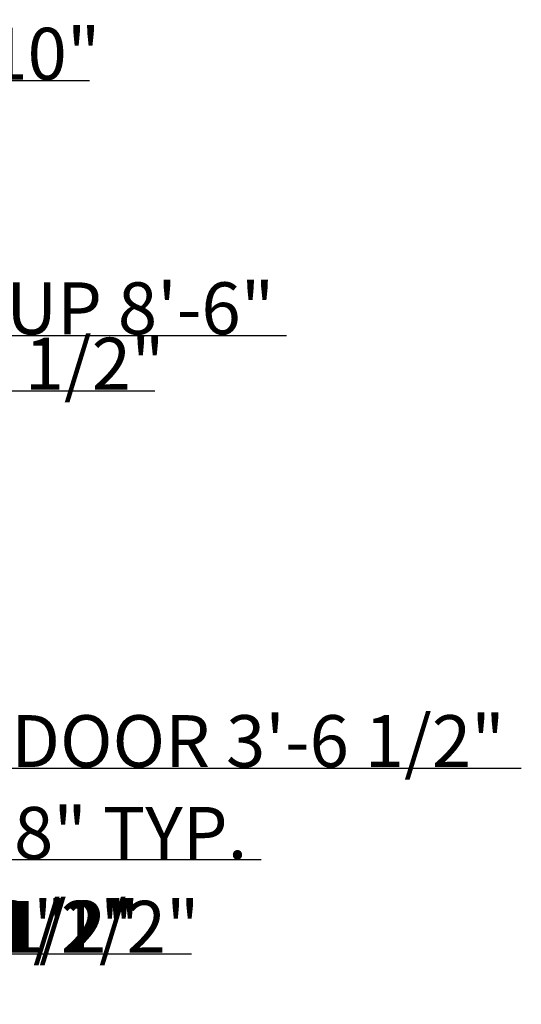
# Model space of a CAD drawing. Units: inches. Extents: x 2236 to 2927, y 1577 to 2452.
# Tile 8 of 9: x 2695 to 2927, y 1679 to 2134. Entities that reach past the tile are written whole.
import ezdxf

# ---------------------------------------------------------------- set-up
doc = ezdxf.new("R2010")
doc.units = ezdxf.units.IN
doc.layers.add('A-ANNO-DIMS', color=2, linetype='Continuous', lineweight=18)
doc.styles.get("Standard").update_dxf_attribs({"font": 'arial.ttf'})
doc.dimstyles.get("Standard").update_dxf_attribs({"dimtxt": 24, "dimasz": 12, "dimexe": 0.18, "dimexo": 0.0625, "dimgap": 0.09, "dimtad": 1, "dimdec": 1, "dimzin": 0, "dimdsep": 46, "dimlunit": 4, "dimtxsty": 'Standard', "dimcen": 0.09, "dimadec": 0, "dimazin": 0, "dimtfac": 1, "dimtdec": 1, "dimtofl": 0, "dimtmove": 0, "dimatfit": 3, "dimfxl": 1, "dimtolj": 1, "dimtzin": 0, "dimarcsym": 0})

# ---------------------------------------------------------------- blocks, each defined once
blk = doc.blocks.new('*D24')
at = {"layer": 'A-ANNO-DIMS', "color": 0, "lineweight": -2, "transparency": 16777216}
for p, q in [((2478.46, 1747), (2478.46, 1745.71)), ((2486.29, 1747), (2486.29, 1745.71)), ((2466.46, 1745.89), (2454.46, 1745.89)), ((2498.29, 1745.89), (2806.59, 1745.89))]:
    blk.add_line(p, q, dxfattribs=at)
at = {"layer": 'A-ANNO-DIMS', "color": 0, "transparency": 16777216}
for points in [[(2466.46, 1747.89), (2466.46, 1743.89), (2478.46, 1745.89)], [(2498.29, 1747.89), (2498.29, 1743.89), (2486.29, 1745.89)]]:
    blk.add_solid(points, dxfattribs=at)
at = {"layer": 'Defpoints', "color": 0, "transparency": 16777216}
for p in [(2478.46, 1747.06), (2486.29, 1747.06), (2486.29, 1745.89)]:
    blk.add_point(p, dxfattribs=at)
at = {"layer": 'A-ANNO-DIMS', "color": 0, "transparency": 16777216, "insert": (2658.44, 1758.23), "char_height": 24, "attachment_point": 5}
blk.add_mtext('\\A1;BURNER 0\'-8" TYP.', dxfattribs=at)
blk = doc.blocks.new('*D27')
at = {"layer": 'A-ANNO-DIMS', "color": 0, "lineweight": -2, "transparency": 16777216}
for p, q in [((2591.96, 1962.5), (2579.96, 1962.5)), ((2603.96, 1964.26), (2603.96, 1962.32)), ((2613.58, 1964.26), (2613.58, 1962.32)), ((2625.58, 1962.5), (2757.48, 1962.5))]:
    blk.add_line(p, q, dxfattribs=at)
at = {"layer": 'A-ANNO-DIMS', "color": 0, "transparency": 16777216}
for points in [[(2591.96, 1964.5), (2591.96, 1960.5), (2603.96, 1962.5)], [(2625.58, 1964.5), (2625.58, 1960.5), (2613.58, 1962.5)]]:
    blk.add_solid(points, dxfattribs=at)
at = {"layer": 'Defpoints', "color": 0, "transparency": 16777216}
for p in [(2603.96, 1964.32), (2613.58, 1964.32), (2613.58, 1962.5)]:
    blk.add_point(p, dxfattribs=at)
at = {"layer": 'A-ANNO-DIMS', "color": 0, "transparency": 16777216, "insert": (2697.53, 1975), "char_height": 24, "attachment_point": 5}
blk.add_mtext('\\A1;0\'-9 1/2"', dxfattribs=at)
blk = doc.blocks.new('*D28')
at = {"layer": 'A-ANNO-DIMS', "color": 0, "lineweight": -2, "transparency": 16777216}
for p, q in [((2430.9, 2003.29), (2430.9, 1987.89)), ((2532.8, 2003.29), (2532.8, 1987.89)), ((2442.9, 1988.07), (2520.8, 1988.07)), ((2532.8, 1988.07), (2818.23, 1988.07))]:
    blk.add_line(p, q, dxfattribs=at)
at = {"layer": 'A-ANNO-DIMS', "color": 0, "transparency": 16777216}
for points in [[(2442.9, 1990.07), (2442.9, 1986.07), (2430.9, 1988.07)], [(2520.8, 1990.07), (2520.8, 1986.07), (2532.8, 1988.07)]]:
    blk.add_solid(points, dxfattribs=at)
at = {"layer": 'Defpoints', "color": 0, "transparency": 16777216}
for p in [(2430.9, 2003.35), (2532.8, 2003.35), (2532.8, 1988.07)]:
    blk.add_point(p, dxfattribs=at)
at = {"layer": 'A-ANNO-DIMS', "color": 0, "transparency": 16777216, "insert": (2681.51, 2000.57), "char_height": 24, "attachment_point": 5}
blk.add_mtext('\\A1;BED GROUP 8\'-6"', dxfattribs=at)
blk = doc.blocks.new('*D34')
at = {"layer": 'A-ANNO-DIMS', "color": 0, "lineweight": -2, "transparency": 16777216}
for p, q in [((2520.69, 1794.44), (2520.69, 1787.92)), ((2563.35, 1794.44), (2563.35, 1787.92)), ((2532.69, 1788.1), (2551.35, 1788.1)), ((2563.35, 1788.1), (2926.83, 1788.1))]:
    blk.add_line(p, q, dxfattribs=at)
at = {"layer": 'A-ANNO-DIMS', "color": 0, "transparency": 16777216}
for points in [[(2532.69, 1790.1), (2532.69, 1786.1), (2520.69, 1788.1)], [(2551.35, 1790.1), (2551.35, 1786.1), (2563.35, 1788.1)]]:
    blk.add_solid(points, dxfattribs=at)
at = {"layer": 'Defpoints', "color": 0, "transparency": 16777216}
for p in [(2520.69, 1794.5), (2563.35, 1794.5), (2563.35, 1788.1)]:
    blk.add_point(p, dxfattribs=at)
at = {"layer": 'A-ANNO-DIMS', "color": 0, "transparency": 16777216, "insert": (2751.09, 1800.62), "char_height": 24, "attachment_point": 5}
blk.add_mtext('\\A1;ENTRY DOOR 3\'-6 1/2"', dxfattribs=at)
blk = doc.blocks.new('*D41')
at = {"layer": 'A-ANNO-DIMS', "color": 0, "lineweight": -2, "transparency": 16777216}
for p, q in [((2588.85, 2105.83), (2576.85, 2105.83)), ((2600.85, 2084.14), (2600.85, 2106.01)), ((2622.85, 2084.14), (2622.85, 2106.01)), ((2634.85, 2105.83), (2727.21, 2105.83))]:
    blk.add_line(p, q, dxfattribs=at)
at = {"layer": 'A-ANNO-DIMS', "color": 0, "transparency": 16777216}
for points in [[(2588.85, 2107.83), (2588.85, 2103.83), (2600.85, 2105.83)], [(2634.85, 2107.83), (2634.85, 2103.83), (2622.85, 2105.83)]]:
    blk.add_solid(points, dxfattribs=at)
at = {"layer": 'Defpoints', "color": 0, "transparency": 16777216}
for p in [(2622.85, 2105.83), (2600.85, 2084.08), (2622.85, 2084.08)]:
    blk.add_point(p, dxfattribs=at)
at = {"layer": 'A-ANNO-DIMS', "color": 0, "transparency": 16777216, "insert": (2687.03, 2118.17), "char_height": 24, "attachment_point": 5}
blk.add_mtext('\\A1;1\'-10"', dxfattribs=at)
blk = doc.blocks.new('*D50')
at = {"layer": 'A-ANNO-DIMS', "color": 0, "lineweight": -2, "transparency": 16777216}
for p, q in [((2563.35, 1793.01), (2563.35, 1702.15)), ((2622.85, 1793.01), (2622.85, 1702.15)), ((2575.35, 1702.33), (2610.85, 1702.33)), ((2622.85, 1702.33), (2774.36, 1702.33))]:
    blk.add_line(p, q, dxfattribs=at)
at = {"layer": 'A-ANNO-DIMS', "color": 0, "transparency": 16777216}
for points in [[(2575.35, 1704.33), (2575.35, 1700.33), (2563.35, 1702.33)], [(2610.85, 1704.33), (2610.85, 1700.33), (2622.85, 1702.33)]]:
    blk.add_solid(points, dxfattribs=at)
at = {"layer": 'Defpoints', "color": 0, "transparency": 16777216}
for p in [(2563.35, 1793.08), (2622.85, 1793.08), (2622.85, 1702.33)]:
    blk.add_point(p, dxfattribs=at)
at = {"layer": 'A-ANNO-DIMS', "color": 0, "transparency": 16777216, "insert": (2704.61, 1714.83), "char_height": 24, "attachment_point": 5}
blk.add_mtext('\\A1;4\'-11 1/2"', dxfattribs=at)
blk = doc.blocks.new('*D55')
at = {"layer": 'A-ANNO-DIMS', "color": 0, "lineweight": -2, "transparency": 16777216}
for p, q in [((2582.18, 1986.01), (2582.18, 1702.15)), ((2613.85, 1986.01), (2613.85, 1702.15)), ((2594.18, 1702.33), (2601.85, 1702.33)), ((2613.85, 1702.33), (2746.16, 1702.33))]:
    blk.add_line(p, q, dxfattribs=at)
at = {"layer": 'A-ANNO-DIMS', "color": 0, "transparency": 16777216}
for points in [[(2594.18, 1704.33), (2594.18, 1700.33), (2582.18, 1702.33)], [(2601.85, 1704.33), (2601.85, 1700.33), (2613.85, 1702.33)]]:
    blk.add_solid(points, dxfattribs=at)
at = {"layer": 'Defpoints', "color": 0, "transparency": 16777216}
for p in [(2582.18, 1986.08), (2613.85, 1986.08), (2613.85, 1702.33)]:
    blk.add_point(p, dxfattribs=at)
at = {"layer": 'A-ANNO-DIMS', "color": 0, "transparency": 16777216, "insert": (2686, 1714.83), "char_height": 24, "attachment_point": 5}
blk.add_mtext('\\A1;2\'-7 1/2"', dxfattribs=at)
blk = doc.blocks.new('*D56')
at = {"layer": 'A-ANNO-DIMS', "color": 0, "lineweight": -2, "transparency": 16777216}
for p, q in [((2551.88, 1874.28), (2551.88, 1702.15)), ((2569.42, 1874.28), (2569.42, 1702.15)), ((2539.88, 1702.33), (2527.88, 1702.33)), ((2581.42, 1702.33), (2711.06, 1702.33))]:
    blk.add_line(p, q, dxfattribs=at)
at = {"layer": 'A-ANNO-DIMS', "color": 0, "transparency": 16777216}
for points in [[(2539.88, 1704.33), (2539.88, 1700.33), (2551.88, 1702.33)], [(2581.42, 1704.33), (2581.42, 1700.33), (2569.42, 1702.33)]]:
    blk.add_solid(points, dxfattribs=at)
at = {"layer": 'Defpoints', "color": 0, "transparency": 16777216}
for p in [(2551.88, 1874.34), (2569.42, 1874.34), (2569.42, 1702.33)]:
    blk.add_point(p, dxfattribs=at)
at = {"layer": 'A-ANNO-DIMS', "color": 0, "transparency": 16777216, "insert": (2652.24, 1714.83), "char_height": 24, "attachment_point": 5}
blk.add_mtext('\\A1;1\'-5 1/2"', dxfattribs=at)
blk = doc.blocks.new('*D64')
at = {"layer": 'A-ANNO-DIMS', "color": 0, "lineweight": -2, "transparency": 16777216}
for p, q in [((2569.42, 1874.28), (2569.42, 1702.15)), ((2580.85, 1860.01), (2580.85, 1702.15)), ((2557.42, 1702.33), (2545.42, 1702.33)), ((2592.85, 1702.33), (2743.4, 1702.33))]:
    blk.add_line(p, q, dxfattribs=at)
at = {"layer": 'A-ANNO-DIMS', "color": 0, "transparency": 16777216}
for points in [[(2557.42, 1704.33), (2557.42, 1700.33), (2569.42, 1702.33)], [(2592.85, 1704.33), (2592.85, 1700.33), (2580.85, 1702.33)]]:
    blk.add_solid(points, dxfattribs=at)
at = {"layer": 'Defpoints', "color": 0, "transparency": 16777216}
for p in [(2569.42, 1874.34), (2580.85, 1860.08), (2580.85, 1702.33)]:
    blk.add_point(p, dxfattribs=at)
at = {"layer": 'A-ANNO-DIMS', "color": 0, "transparency": 16777216, "insert": (2674.12, 1714.83), "char_height": 24, "attachment_point": 5}
blk.add_mtext('\\A1;0\'-11 1/2"', dxfattribs=at)

msp = doc.modelspace()

# ---------------------------------------------------------------- dimensions: what is measured, and where the dimension line sits
at = {"layer": 'A-ANNO-DIMS'}
for base, p1, p2, picture, middle in [((2622.85, 2105.83), (2600.85, 2084.08), (2622.85, 2084.08), '*D41', (2687.03, 2118.17)), ((2613.58, 1962.5), (2603.96, 1964.32), (2613.58, 1964.32), '*D27', (2697.53, 1975)), ((2613.85, 1702.33), (2582.18, 1986.08), (2613.85, 1986.08), '*D55', (2686, 1714.83)), ((2569.42, 1702.33), (2551.88, 1874.34), (2569.42, 1874.34), '*D56', (2652.24, 1714.83)), ((2580.85, 1702.33), (2569.42, 1874.34), (2580.85, 1860.08), '*D64', (2674.12, 1714.83)), ((2622.85, 1702.33), (2563.35, 1793.08), (2622.85, 1793.08), '*D50', (2704.61, 1714.83))]:
    dim = msp.add_linear_dim(base=base, p1=p1, p2=p2, dimstyle='Standard', override={"dimdec": 1, "dimlfac": 1, "dimrnd": 0, "dimzin": 1, "dimdsep": 46, "dimlunit": 4, "dimfrac": 2}, dxfattribs=at)
    dim.commit()
    dim.dimension.update_dxf_attribs({"geometry": picture, "text_midpoint": middle})
for base, p1, p2, text, picture, middle in [((2532.8, 1988.07), (2430.9, 2003.35), (2532.8, 2003.35), 'BED GROUP <>', '*D28', (2681.51, 2000.57)), ((2563.35, 1788.1), (2520.69, 1794.5), (2563.35, 1794.5), 'ENTRY DOOR <>', '*D34', (2751.09, 1800.62)), ((2486.29, 1745.89), (2478.46, 1747.06), (2486.29, 1747.06), 'BURNER <> TYP.', '*D24', (2658.44, 1758.23))]:
    dim = msp.add_linear_dim(base=base, p1=p1, p2=p2, text=text, dimstyle='Standard', override={"dimdec": 1, "dimlfac": 1, "dimrnd": 0, "dimzin": 1, "dimdsep": 46, "dimlunit": 4, "dimfrac": 2}, dxfattribs=at)
    dim.commit()
    dim.dimension.update_dxf_attribs({"geometry": picture, "text_midpoint": middle})

doc.saveas('drawing.dxf')
